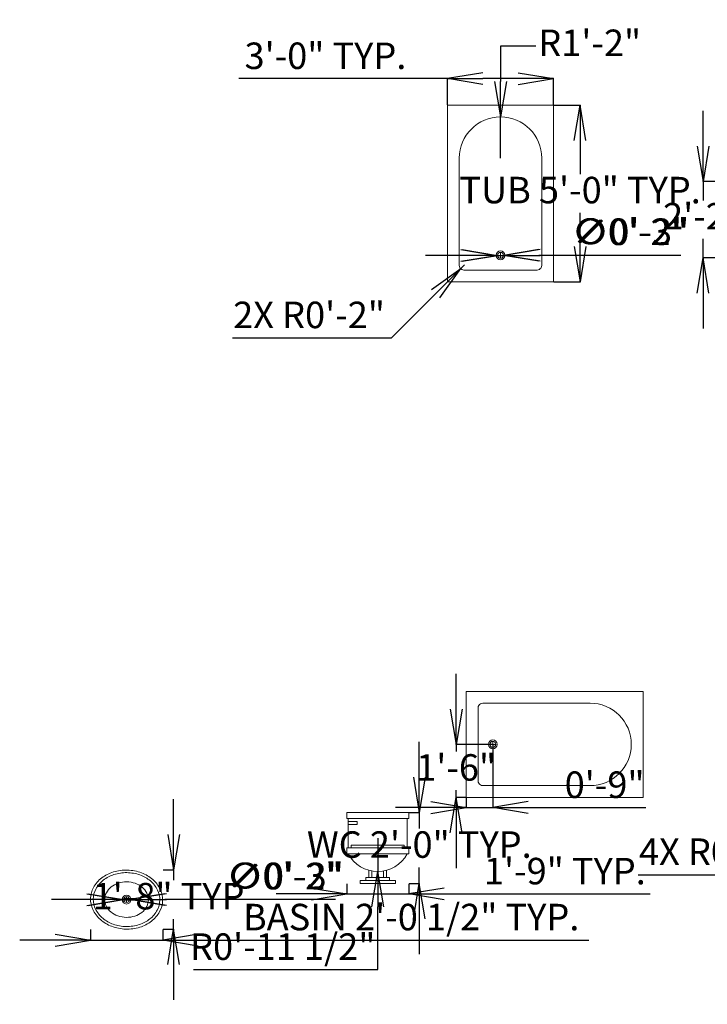
# Model space of a CAD drawing. Units: inches. Extents: x 1856 to 3350, y 1624 to 2224.
# Tile 4 of 7: x 2521 to 2754, y 1634 to 1968. Entities that reach past the tile are written whole.
import ezdxf

# ---------------------------------------------------------------- set-up
doc = ezdxf.new("R2010")
doc.units = ezdxf.units.IN
doc.layers.add('A-ANNO-DIMS', color=2, linetype='Continuous', lineweight=18)
doc.layers.add('A-FLOR-FIXT', color=3, linetype='Continuous', lineweight=18)
doc.styles.get("Standard").update_dxf_attribs({"font": 'arial.ttf'})
doc.dimstyles.new('ISO-25', dxfattribs={"dimtxt": 9, "dimasz": 12, "dimexe": 0.125, "dimexo": 0.125, "dimgap": 2, "dimtad": 1, "dimtih": 1, "dimtoh": 1, "dimdec": 1, "dimzin": 11, "dimlunit": 4, "dimtxsty": 'Standard', "dimblk": 'OPEN', "dimcen": -0.125, "dimadec": 0, "dimazin": 0, "dimtfac": 1, "dimtdec": 1, "dimtmove": 0, "dimatfit": 3, "dimfxl": 1, "dimarcsym": 0})

# ---------------------------------------------------------------- blocks, each defined once
blk = doc.blocks.new('Toilet - front')
for p, q in [((-10, 22), (-10, 12)), ((-10, 21), (-7, 21)), ((-7, 21), (-7, 20)), ((10, 12), (10, 22)), ((-7, 20), (-10, 20)), ((10.5, 12), (-10.5, 12)), ((-10.5, 10), (-10.5, 12)), ((9, 13), (-9, 13)), ((-9, 13), (-9, 12)), ((9, 12), (9, 13)), ((10.5, 12), (10.5, 10)), ((10.5, 10), (-10.5, 10)), ((-3, 4.4065), (-3, 2)), ((-2, 2), (-2, 4.1658)), ((2, 4.1658), (2, 2)), ((3, 2), (3, 4.4065)), ((4, 2), (-4, 2)), ((-4, 2), (-4, 1)), ((4, 1), (4, 2))]:
    blk.add_line(p, q)
for points in [[(10.5, 22), (10.5, 24), (-10.5, 24), (-10.5, 22)], [(6, 0), (6, 1), (-6, 1), (-6, 0)]]:
    blk.add_lwpolyline(points, close=True)
blk.add_arc((0, 15.3333), 11.3333, 208.0725, 331.9275)
blk = doc.blocks.new('Sink - Oval top')
for p, q in [((-1, 0), (1, 0)), ((0, 1), (0, -1))]:
    blk.add_line(p, q)
for points in [[(-12.23, 0.39, 0.117634), (-11.46, -3.36, 0.104469), (-8.88, -6.8, 0.090016), (-5.08, -9.07, 0.08192), (-0.32, -10.02, 0.08192), (4.49, -9.38, 0.090016), (8.42, -7.36, 0.104469), (11.22, -4.09, 0.117634), (12.23, -0.39, 0.117634), (11.46, 3.36, 0.104469), (8.88, 6.8, 0.090016), (5.08, 9.07, 0.08192), (0.32, 10.02, 0.08192), (-4.49, 9.38, 0.090016), (-8.42, 7.36, 0.104469), (-11.22, 4.09, 0.117634)], [(-11.29, 0.16, 0.118622), (-10.52, -3.25, 0.104678), (-8.07, -6.36, 0.089562), (-4.54, -8.37, 0.081185), (-0.13, -9.15, 0.081185), (4.3, -8.49, 0.089562), (7.89, -6.58, 0.104678), (10.42, -3.55, 0.118622), (11.29, -0.16, 0.118622), (10.52, 3.25, 0.104678), (8.07, 6.36, 0.089562), (4.54, 8.37, 0.081185), (0.13, 9.15, 0.081185), (-4.3, 8.49, 0.089562), (-7.89, 6.58, 0.104678), (-10.42, 3.55, 0.118622)], [(-7.42, 0.08, 0.118283), (-6.91, -2.17, 0.104607), (-5.29, -4.21, 0.089718), (-2.97, -5.53, 0.081436), (-0.07, -6.04, 0.081436), (2.84, -5.59, 0.089718), (5.2, -4.33, 0.104607), (6.86, -2.32, 0.118283), (7.42, -0.08, 0.118283), (6.91, 2.17, 0.104607), (5.29, 4.21, 0.089718), (2.97, 5.53, 0.081436), (0.07, 6.04, 0.081436), (-2.84, 5.59, 0.089718), (-5.2, 4.33, 0.104607), (-6.86, 2.32, 0.118283)]]:
    blk.add_lwpolyline(points, format="xyb", close=True)
for radius in [1.5, 1]:
    blk.add_circle((0, 0), radius)
blk = doc.blocks.new('Bath Tub - 26 x 60 in.')
for p, q in [((8, -18), (10, -18)), ((9, -17), (9, -19))]:
    blk.add_line(p, q)
blk.add_lwpolyline([(0, -36), (0, 0), (60, 0), (60, -36)], close=True)
for points in [[(4, -30), (4, -6)], [(6, -4), (42, -4)], [(42, -32), (6, -32)]]:
    blk.add_lwpolyline(points)
for radius in [1.5, 1]:
    blk.add_circle((9, -18), radius)
for centre, radius, start, end in [((5.75, -5.75), 1.77, 81.8699, 188.1301), ((42, -18), 14, 270, 90), ((5.75, -30.25), 1.77, 171.8699, 278.1301)]:
    blk.add_arc(centre, radius, start, end)
blk = doc.blocks.new('_Open')
at = {"color": 0, "linetype": 'ByBlock', "lineweight": -2}
for p, q in [((-1, 0.167), (0, 0)), ((-1, -0.167), (0, 0)), ((0, 0), (-1, 0))]:
    blk.add_line(p, q, dxfattribs=at)
blk = doc.blocks.new('*D50')
at = {"layer": 'A-ANNO-DIMS', "color": 0, "lineweight": -2, "transparency": 16777216}
for p, q in [((2545.08, 1659.26), (2545.08, 1655.58)), ((2569.63, 1659.26), (2569.63, 1655.58)), ((2533.08, 1655.7), (2521.08, 1655.7)), ((2545.08, 1655.7), (2569.63, 1655.7)), ((2581.63, 1655.7), (2714.29, 1655.7))]:
    blk.add_line(p, q, dxfattribs=at)
at = {"layer": 'Defpoints', "color": 0, "transparency": 16777216}
for p in [(2545.08, 1659.39), (2569.63, 1659.39), (2569.63, 1655.7)]:
    blk.add_point(p, dxfattribs=at)
at = {"layer": 'A-ANNO-DIMS', "color": 0, "lineweight": -2, "transparency": 16777216, "xscale": 12, "yscale": 12, "zscale": 12}
blk.add_blockref('_Open', (2545.08, 1655.7), dxfattribs=at)
at = {"layer": 'A-ANNO-DIMS', "color": 0, "lineweight": -2, "transparency": 16777216, "xscale": 12, "yscale": 12, "zscale": 12, "rotation": 180}
blk.add_blockref('_Open', (2569.63, 1655.7), dxfattribs=at)
at = {"layer": 'A-ANNO-DIMS', "color": 0, "transparency": 16777216, "insert": (2653.96, 1662.36), "char_height": 9, "attachment_point": 5}
blk.add_mtext('BASIN 2\'-0 1/2" TYP.', dxfattribs=at)
blk = doc.blocks.new('*D51')
at = {"layer": 'A-ANNO-DIMS', "color": 0, "lineweight": -2, "transparency": 16777216}
for p, q in [((2573.32, 1691.52), (2573.32, 1703.52)), ((2569.76, 1679.52), (2573.44, 1679.52)), ((2573.32, 1679.52), (2573.32, 1676.05)), ((2573.32, 1659.39), (2573.32, 1662.86)), ((2569.76, 1659.39), (2573.44, 1659.39)), ((2573.32, 1647.39), (2573.32, 1635.39))]:
    blk.add_line(p, q, dxfattribs=at)
at = {"layer": 'Defpoints', "color": 0, "transparency": 16777216}
for p in [(2569.63, 1679.52), (2573.32, 1679.52), (2569.63, 1659.39)]:
    blk.add_point(p, dxfattribs=at)
at = {"layer": 'A-ANNO-DIMS', "color": 0, "lineweight": -2, "transparency": 16777216, "xscale": 12, "yscale": 12, "zscale": 12}
for p, rotation in [((2573.32, 1679.52), 270), ((2573.32, 1659.39), 90)]:
    blk.add_blockref('_Open', p, dxfattribs=dict(at, rotation=rotation))
at = {"layer": 'A-ANNO-DIMS', "color": 0, "transparency": 16777216, "insert": (2573.32, 1669.46), "char_height": 9, "attachment_point": 5}
blk.add_mtext('1\'-8" TYP.', dxfattribs=at)
blk = doc.blocks.new('*D52')
at = {"layer": 'A-ANNO-DIMS', "color": 0, "lineweight": -2, "transparency": 16777216}
for p, q in [((2656.73, 1710.98), (2656.73, 1722.98)), ((2653.25, 1698.98), (2656.85, 1698.98)), ((2656.73, 1698.98), (2656.73, 1693.63)), ((2656.73, 1674.98), (2656.73, 1680.32)), ((2653.25, 1674.98), (2656.85, 1674.98)), ((2656.73, 1662.98), (2656.73, 1650.98))]:
    blk.add_line(p, q, dxfattribs=at)
at = {"layer": 'Defpoints', "color": 0, "transparency": 16777216}
for p in [(2653.13, 1698.98), (2656.73, 1698.98), (2653.13, 1674.98)]:
    blk.add_point(p, dxfattribs=at)
at = {"layer": 'A-ANNO-DIMS', "color": 0, "lineweight": -2, "transparency": 16777216, "xscale": 12, "yscale": 12, "zscale": 12}
for p, rotation in [((2656.73, 1698.98), 270), ((2656.73, 1674.98), 90)]:
    blk.add_blockref('_Open', p, dxfattribs=dict(at, rotation=rotation))
at = {"layer": 'A-ANNO-DIMS', "color": 0, "transparency": 16777216, "insert": (2656.73, 1686.98), "char_height": 9, "attachment_point": 5}
blk.add_mtext('WC 2\'-0" TYP.', dxfattribs=at)
blk = doc.blocks.new('*D53')
at = {"layer": 'A-ANNO-DIMS', "color": 0, "lineweight": -2, "transparency": 16777216}
for p, q in [((2632.13, 1674.85), (2632.13, 1671.25)), ((2653.13, 1674.85), (2653.13, 1671.25)), ((2620.13, 1671.38), (2608.13, 1671.38)), ((2632.13, 1671.38), (2653.13, 1671.38)), ((2665.13, 1671.38), (2735.14, 1671.38))]:
    blk.add_line(p, q, dxfattribs=at)
at = {"layer": 'Defpoints', "color": 0, "transparency": 16777216}
for p in [(2632.13, 1674.98), (2653.13, 1674.98), (2653.13, 1671.38)]:
    blk.add_point(p, dxfattribs=at)
at = {"layer": 'A-ANNO-DIMS', "color": 0, "lineweight": -2, "transparency": 16777216, "xscale": 12, "yscale": 12, "zscale": 12}
blk.add_blockref('_Open', (2632.13, 1671.38), dxfattribs=at)
at = {"layer": 'A-ANNO-DIMS', "color": 0, "lineweight": -2, "transparency": 16777216, "xscale": 12, "yscale": 12, "zscale": 12, "rotation": 180}
blk.add_blockref('_Open', (2653.13, 1671.38), dxfattribs=at)
at = {"layer": 'A-ANNO-DIMS', "color": 0, "transparency": 16777216, "insert": (2706.14, 1677.97), "char_height": 9, "attachment_point": 5}
blk.add_mtext('1\'-9" TYP.', dxfattribs=at)
blk = doc.blocks.new('*D54')
at = {"layer": 'A-ANNO-DIMS', "color": 0, "lineweight": -2, "transparency": 16777216}
for p, q in [((2702.42, 1939.19), (2711.42, 1939.19)), ((2711.3, 1927.19), (2711.3, 1915.79)), ((2711.3, 1891.19), (2711.3, 1902.59)), ((2702.42, 1879.19), (2711.42, 1879.19))]:
    blk.add_line(p, q, dxfattribs=at)
at = {"layer": 'Defpoints', "color": 0, "transparency": 16777216}
for p in [(2702.3, 1939.19), (2711.3, 1939.19), (2702.3, 1879.19)]:
    blk.add_point(p, dxfattribs=at)
at = {"layer": 'A-ANNO-DIMS', "color": 0, "lineweight": -2, "transparency": 16777216, "xscale": 12, "yscale": 12, "zscale": 12}
for p, rotation in [((2711.3, 1939.19), 90), ((2711.3, 1879.19), 270)]:
    blk.add_blockref('_Open', p, dxfattribs=dict(at, rotation=rotation))
at = {"layer": 'A-ANNO-DIMS', "color": 0, "transparency": 16777216, "insert": (2711.3, 1909.19), "char_height": 9, "attachment_point": 5}
blk.add_mtext('TUB 5\'-0" TYP.', dxfattribs=at)
blk = doc.blocks.new('*D55')
at = {"layer": 'A-ANNO-DIMS', "color": 0, "lineweight": -2, "transparency": 16777216}
for p, q in [((2666.3, 1948.19), (2595.44, 1948.19)), ((2666.3, 1939.31), (2666.3, 1948.31)), ((2690.3, 1948.19), (2678.3, 1948.19)), ((2702.3, 1939.31), (2702.3, 1948.31))]:
    blk.add_line(p, q, dxfattribs=at)
at = {"layer": 'Defpoints', "color": 0, "transparency": 16777216}
for p in [(2666.3, 1948.19), (2666.3, 1939.19), (2702.3, 1939.19)]:
    blk.add_point(p, dxfattribs=at)
at = {"layer": 'A-ANNO-DIMS', "color": 0, "lineweight": -2, "transparency": 16777216, "xscale": 12, "yscale": 12, "zscale": 12, "rotation": 180}
blk.add_blockref('_Open', (2666.3, 1948.19), dxfattribs=at)
at = {"layer": 'A-ANNO-DIMS', "color": 0, "lineweight": -2, "transparency": 16777216, "xscale": 12, "yscale": 12, "zscale": 12}
blk.add_blockref('_Open', (2702.3, 1948.19), dxfattribs=at)
at = {"layer": 'A-ANNO-DIMS', "color": 0, "transparency": 16777216, "insert": (2624.87, 1954.79), "char_height": 9, "attachment_point": 5}
blk.add_mtext('3\'-0" TYP.', dxfattribs=at)
blk = doc.blocks.new('*D76')
at = {"layer": 'A-ANNO-DIMS', "color": 0, "lineweight": -2, "transparency": 16777216}
for p, q in [((2753.05, 1925.32), (2753.05, 1937.32)), ((2757.48, 1913.32), (2752.93, 1913.32)), ((2753.05, 1913.32), (2753.05, 1906.83)), ((2753.05, 1887.32), (2753.05, 1893.8)), ((2757.48, 1887.32), (2752.93, 1887.32)), ((2753.05, 1875.32), (2753.05, 1863.32))]:
    blk.add_line(p, q, dxfattribs=at)
at = {"layer": 'Defpoints', "color": 0, "transparency": 16777216}
for p in [(2757.6, 1913.32), (2753.05, 1887.32), (2757.6, 1887.32)]:
    blk.add_point(p, dxfattribs=at)
at = {"layer": 'A-ANNO-DIMS', "color": 0, "lineweight": -2, "transparency": 16777216, "xscale": 12, "yscale": 12, "zscale": 12}
for p, rotation in [((2753.05, 1913.32), 270), ((2753.05, 1887.32), 90)]:
    blk.add_blockref('_Open', p, dxfattribs=dict(at, rotation=rotation))
at = {"layer": 'A-ANNO-DIMS', "color": 0, "transparency": 16777216, "insert": (2753.05, 1900.32), "char_height": 9, "attachment_point": 5}
blk.add_mtext('2\'-2"', dxfattribs=at)
blk = doc.blocks.new('*D87')
at = {"layer": 'A-ANNO-DIMS', "color": 0, "lineweight": -2, "transparency": 16777216}
for p, q in [((2681.68, 1722.03), (2681.68, 1700.58)), ((2672.68, 1704.03), (2672.68, 1700.58)), ((2660.68, 1700.71), (2648.68, 1700.71)), ((2672.68, 1700.71), (2681.68, 1700.71)), ((2693.68, 1700.71), (2733.6, 1700.71))]:
    blk.add_line(p, q, dxfattribs=at)
at = {"layer": 'Defpoints', "color": 0, "transparency": 16777216}
for p in [(2681.68, 1722.16), (2672.68, 1704.16), (2681.68, 1700.71)]:
    blk.add_point(p, dxfattribs=at)
at = {"layer": 'A-ANNO-DIMS', "color": 0, "lineweight": -2, "transparency": 16777216, "xscale": 12, "yscale": 12, "zscale": 12}
blk.add_blockref('_Open', (2672.68, 1700.71), dxfattribs=at)
at = {"layer": 'A-ANNO-DIMS', "color": 0, "lineweight": -2, "transparency": 16777216, "xscale": 12, "yscale": 12, "zscale": 12, "rotation": 180}
blk.add_blockref('_Open', (2681.68, 1700.71), dxfattribs=at)
at = {"layer": 'A-ANNO-DIMS', "color": 0, "transparency": 16777216, "insert": (2719.64, 1707.3), "char_height": 9, "attachment_point": 5}
blk.add_mtext('0\'-9"', dxfattribs=at)
blk = doc.blocks.new('*D88')
at = {"layer": 'A-ANNO-DIMS', "color": 0, "lineweight": -2, "transparency": 16777216}
for p, q in [((2669.23, 1734.16), (2669.23, 1746.16)), ((2681.55, 1722.16), (2669.1, 1722.16)), ((2669.23, 1722.16), (2669.23, 1719.75)), ((2669.23, 1704.16), (2669.23, 1706.56)), ((2672.55, 1704.16), (2669.1, 1704.16)), ((2669.23, 1692.16), (2669.23, 1680.16))]:
    blk.add_line(p, q, dxfattribs=at)
at = {"layer": 'Defpoints', "color": 0, "transparency": 16777216}
for p in [(2669.23, 1722.16), (2681.68, 1722.16), (2672.68, 1704.16)]:
    blk.add_point(p, dxfattribs=at)
at = {"layer": 'A-ANNO-DIMS', "color": 0, "lineweight": -2, "transparency": 16777216, "xscale": 12, "yscale": 12, "zscale": 12}
for p, rotation in [((2669.23, 1722.16), 270), ((2669.23, 1704.16), 90)]:
    blk.add_blockref('_Open', p, dxfattribs=dict(at, rotation=rotation))
at = {"layer": 'A-ANNO-DIMS', "color": 0, "transparency": 16777216, "insert": (2669.23, 1713.16), "char_height": 9, "attachment_point": 5}
blk.add_mtext('1\'-6"', dxfattribs=at)
blk = doc.blocks.new('*D101')
at = {"layer": 'A-ANNO-DIMS', "color": 0, "lineweight": -2, "transparency": 16777216}
for p, q in [((2830.88, 1702.51), (2829.82, 1701.45)), ((2806.26, 1677.9), (2821.33, 1692.97)), ((2731.06, 1677.9), (2806.26, 1677.9))]:
    blk.add_line(p, q, dxfattribs=at)
at = {"layer": 'Defpoints', "color": 0, "transparency": 16777216}
for p in [(2830.88, 1702.51), (2829.82, 1701.45)]:
    blk.add_point(p, dxfattribs=at)
at = {"layer": 'A-ANNO-DIMS', "color": 0, "lineweight": -2, "transparency": 16777216, "xscale": 12, "yscale": 12, "zscale": 12, "rotation": 44.99157303797349}
blk.add_blockref('_Open', (2829.82, 1701.45), dxfattribs=at)
at = {"layer": 'A-ANNO-DIMS', "color": 0, "transparency": 16777216, "insert": (2767.66, 1684.56), "char_height": 9, "attachment_point": 5}
blk.add_mtext('4X R0\'-1 1/2"', dxfattribs=at)
blk = doc.blocks.new('*D102')
at = {"layer": 'A-ANNO-DIMS', "color": 0, "lineweight": -2, "transparency": 16777216}
for p, q in [((2696.3, 1959.19), (2684.3, 1959.19)), ((2684.3, 1959.19), (2684.3, 1947.19)), ((2684.3, 1921.19), (2684.3, 1935.19))]:
    blk.add_line(p, q, dxfattribs=at)
at = {"layer": 'Defpoints', "color": 0, "transparency": 16777216}
for p in [(2684.3, 1935.19), (2684.3, 1921.19)]:
    blk.add_point(p, dxfattribs=at)
at = {"layer": 'A-ANNO-DIMS', "color": 0, "lineweight": -2, "transparency": 16777216, "xscale": 12, "yscale": 12, "zscale": 12, "rotation": 269.9990218791928}
blk.add_blockref('_Open', (2684.3, 1935.19), dxfattribs=at)
at = {"layer": 'A-ANNO-DIMS', "color": 0, "transparency": 16777216, "insert": (2714.57, 1959.19), "char_height": 9, "attachment_point": 5}
blk.add_mtext('R1\'-2"', dxfattribs=at)
blk = doc.blocks.new('*D103')
at = {"layer": 'A-ANNO-DIMS', "color": 0, "lineweight": -2, "transparency": 16777216}
for p, q in [((2672.05, 1884.94), (2670.8, 1883.69)), ((2647.33, 1860.22), (2662.31, 1875.2)), ((2593.3, 1860.22), (2647.33, 1860.22))]:
    blk.add_line(p, q, dxfattribs=at)
at = {"layer": 'Defpoints', "color": 0, "transparency": 16777216}
for p in [(2670.8, 1883.69), (2672.05, 1884.94)]:
    blk.add_point(p, dxfattribs=at)
at = {"layer": 'A-ANNO-DIMS', "color": 0, "lineweight": -2, "transparency": 16777216, "xscale": 12, "yscale": 12, "zscale": 12, "rotation": 45.00288770727251}
blk.add_blockref('_Open', (2670.8, 1883.69), dxfattribs=at)
at = {"layer": 'A-ANNO-DIMS', "color": 0, "transparency": 16777216, "insert": (2619.31, 1866.81), "char_height": 9, "attachment_point": 5}
blk.add_mtext('2X R0\'-2"', dxfattribs=at)
blk = doc.blocks.new('*D104')
at = {"layer": 'A-ANNO-DIMS', "color": 0, "lineweight": -2, "transparency": 16777216}
for p, q in [((2670.8, 1888.19), (2658.8, 1888.19)), ((2682.8, 1888.19), (2685.8, 1888.19)), ((2709.8, 1888.19), (2697.8, 1888.19)), ((2745.51, 1888.19), (2709.8, 1888.19))]:
    blk.add_line(p, q, dxfattribs=at)
at = {"layer": 'Defpoints', "color": 0, "transparency": 16777216}
for p in [(2682.8, 1888.19), (2685.8, 1888.19)]:
    blk.add_point(p, dxfattribs=at)
at = {"layer": 'A-ANNO-DIMS', "color": 0, "lineweight": -2, "transparency": 16777216, "xscale": 12, "yscale": 12, "zscale": 12}
for p, rotation in [((2682.8, 1888.19), 0.0043162820506559), ((2685.8, 1888.19), 180.0043162820506)]:
    blk.add_blockref('_Open', p, dxfattribs=dict(at, rotation=rotation))
at = {"layer": 'A-ANNO-DIMS', "color": 0, "transparency": 16777216, "insert": (2728.65, 1895.04), "char_height": 9, "attachment_point": 5}
blk.add_mtext('∅0\'-3"', dxfattribs=at)
blk = doc.blocks.new('*D105')
at = {"layer": 'A-ANNO-DIMS', "color": 0, "lineweight": -2, "transparency": 16777216}
for p, q in [((2671.3, 1888.19), (2659.3, 1888.19)), ((2683.3, 1888.19), (2685.3, 1888.19)), ((2709.3, 1888.19), (2697.3, 1888.19)), ((2745.01, 1888.19), (2709.3, 1888.19))]:
    blk.add_line(p, q, dxfattribs=at)
at = {"layer": 'Defpoints', "color": 0, "transparency": 16777216}
for p in [(2683.3, 1888.19), (2685.3, 1888.19)]:
    blk.add_point(p, dxfattribs=at)
at = {"layer": 'A-ANNO-DIMS', "color": 0, "lineweight": -2, "transparency": 16777216, "xscale": 12, "yscale": 12, "zscale": 12}
for p, rotation in [((2683.3, 1888.19), 0.0064744230541614), ((2685.3, 1888.19), 180.0064744230541)]:
    blk.add_blockref('_Open', p, dxfattribs=dict(at, rotation=rotation))
at = {"layer": 'A-ANNO-DIMS', "color": 0, "transparency": 16777216, "insert": (2728.15, 1895.04), "char_height": 9, "attachment_point": 5}
blk.add_mtext('∅0\'-2"', dxfattribs=at)
blk = doc.blocks.new('*D106')
at = {"layer": 'A-ANNO-DIMS', "color": 0, "lineweight": -2, "transparency": 16777216}
for p, q in [((2642.63, 1690.31), (2642.63, 1678.98)), ((2642.63, 1645.67), (2642.63, 1666.98)), ((2580.13, 1645.67), (2642.63, 1645.67))]:
    blk.add_line(p, q, dxfattribs=at)
at = {"layer": 'Defpoints', "color": 0, "transparency": 16777216}
for p in [(2642.63, 1690.31), (2642.63, 1678.98)]:
    blk.add_point(p, dxfattribs=at)
at = {"layer": 'A-ANNO-DIMS', "color": 0, "lineweight": -2, "transparency": 16777216, "xscale": 12, "yscale": 12, "zscale": 12, "rotation": 89.99933267248882}
blk.add_blockref('_Open', (2642.63, 1678.98), dxfattribs=at)
at = {"layer": 'A-ANNO-DIMS', "color": 0, "transparency": 16777216, "insert": (2610.38, 1652.32), "char_height": 9, "attachment_point": 5}
blk.add_mtext('R0\'-11 1/2"', dxfattribs=at)
blk = doc.blocks.new('*D107')
at = {"layer": 'A-ANNO-DIMS', "color": 0, "lineweight": -2, "transparency": 16777216}
for p, q in [((2543.86, 1669.46), (2531.86, 1669.46)), ((2555.86, 1669.46), (2558.86, 1669.45)), ((2592.55, 1669.45), (2570.86, 1669.45)), ((2628.27, 1669.45), (2592.55, 1669.45))]:
    blk.add_line(p, q, dxfattribs=at)
at = {"layer": 'Defpoints', "color": 0, "transparency": 16777216}
for p in [(2555.86, 1669.46), (2558.86, 1669.45)]:
    blk.add_point(p, dxfattribs=at)
at = {"layer": 'A-ANNO-DIMS', "color": 0, "lineweight": -2, "transparency": 16777216, "xscale": 12, "yscale": 12, "zscale": 12}
for p, rotation in [((2555.86, 1669.46), 359.985752449785), ((2558.86, 1669.45), 179.9857524497849)]:
    blk.add_blockref('_Open', p, dxfattribs=dict(at, rotation=rotation))
at = {"layer": 'A-ANNO-DIMS', "color": 0, "transparency": 16777216, "insert": (2611.41, 1676.29), "char_height": 9, "attachment_point": 5}
blk.add_mtext('∅0\'-3"', dxfattribs=at)
blk = doc.blocks.new('*D108')
at = {"layer": 'A-ANNO-DIMS', "color": 0, "lineweight": -2, "transparency": 16777216}
for p, q in [((2544.36, 1669.46), (2532.36, 1669.46)), ((2556.36, 1669.46), (2558.36, 1669.45)), ((2592.05, 1669.44), (2570.36, 1669.45)), ((2627.77, 1669.44), (2592.05, 1669.44))]:
    blk.add_line(p, q, dxfattribs=at)
at = {"layer": 'Defpoints', "color": 0, "transparency": 16777216}
for p in [(2556.36, 1669.46), (2558.36, 1669.45)]:
    blk.add_point(p, dxfattribs=at)
at = {"layer": 'A-ANNO-DIMS', "color": 0, "lineweight": -2, "transparency": 16777216, "xscale": 12, "yscale": 12, "zscale": 12}
for p, rotation in [((2556.36, 1669.46), 359.9786286752216), ((2558.36, 1669.45), 179.9786286752215)]:
    blk.add_blockref('_Open', p, dxfattribs=dict(at, rotation=rotation))
at = {"layer": 'A-ANNO-DIMS', "color": 0, "transparency": 16777216, "insert": (2610.91, 1676.29), "char_height": 9, "attachment_point": 5}
blk.add_mtext('∅0\'-2"', dxfattribs=at)

msp = doc.modelspace()

# ---------------------------------------------------------------- block references
at = {"layer": 'A-FLOR-FIXT', "rotation": 90}
msp.add_blockref('Bath Tub - 26 x 60 in.', (2666.3, 1879.19), dxfattribs=at)
at = {"layer": 'A-FLOR-FIXT'}
for name, p in [('Bath Tub - 26 x 60 in.', (2672.68, 1740.16)), ('Toilet - front', (2642.63, 1674.98)), ('Sink - Oval top', (2557.36, 1669.46))]:
    msp.add_blockref(name, p, dxfattribs=at)

# ---------------------------------------------------------------- dimensions: what is measured, and where the dimension line sits
at = {"layer": 'A-ANNO-DIMS'}
for base, p1, p2, angle, text, picture, middle in [((2666.3, 1948.19), (2702.3, 1939.19), (2666.3, 1939.19), 180, '<> TYP.', '*D55', (2624.87, 1954.79)), ((2711.3, 1939.19), (2702.3, 1879.19), (2702.3, 1939.19), 90, 'TUB <> TYP.', '*D54', (2711.3, 1909.19)), ((2656.73, 1698.98), (2653.13, 1674.98), (2653.13, 1698.98), 90, 'WC <> TYP.', '*D52', (2656.73, 1686.98)), ((2573.32, 1679.52), (2569.63, 1659.39), (2569.63, 1679.52), 90, '<> TYP.', '*D51', (2573.32, 1669.46))]:
    dim = msp.add_linear_dim(base=base, p1=p1, p2=p2, angle=angle, text=text, dimstyle='ISO-25', override={"dimdec": 1, "dimlfac": 1, "dimrnd": 0, "dimzin": 1, "dimdsep": 46, "dimlunit": 4, "dimfrac": 2}, dxfattribs=at)
    dim.commit()
    dim.dimension.update_dxf_attribs({"geometry": picture, "text_midpoint": middle})
for center, mpoint, picture, middle in [((2684.3, 1921.19), (2684.3, 1935.19), '*D102', (2714.57, 1959.19)), ((2642.63, 1690.31), (2642.63, 1678.98), '*D106', (2610.38, 1652.32))]:
    dim = msp.add_radius_dim(center=center, mpoint=mpoint, dimstyle='ISO-25', override={"dimdec": 1, "dimlfac": 1, "dimrnd": 0, "dimzin": 1, "dimdsep": 46, "dimlunit": 4, "dimfrac": 2}, dxfattribs=at)
    dim.commit()
    dim.dimension.update_dxf_attribs({"geometry": picture, "text_midpoint": middle})
for base, p1, p2, picture, middle in [((2753.05, 1887.32), (2757.6, 1913.32), (2757.6, 1887.32), '*D76', (2753.05, 1900.32)), ((2669.23, 1722.16), (2672.68, 1704.16), (2681.68, 1722.16), '*D88', (2669.23, 1713.16))]:
    dim = msp.add_linear_dim(base=base, p1=p1, p2=p2, angle=90, dimstyle='ISO-25', override={"dimdec": 1, "dimlfac": 1, "dimrnd": 0, "dimzin": 1, "dimdsep": 46, "dimlunit": 4, "dimfrac": 2}, dxfattribs=at)
    dim.commit()
    dim.dimension.update_dxf_attribs({"geometry": picture, "text_midpoint": middle})
dim = msp.add_diameter_dim_2p(p1=(2682.8, 1888.19), p2=(2685.8, 1888.19), dimstyle='ISO-25', override={"dimdec": 1, "dimlfac": 1, "dimrnd": 0, "dimzin": 1, "dimdsep": 46, "dimlunit": 4, "dimfrac": 2}, dxfattribs=at)
dim.commit()
dim.dimension.update_dxf_attribs({"geometry": '*D104', "text_midpoint": (2709.8, 1888.19), "dimtype": 163})
for p1, p2, picture, middle in [((2683.3, 1888.19), (2685.3, 1888.19), '*D105', (2709.3, 1888.19)), ((2555.86, 1669.46), (2558.86, 1669.45), '*D107', (2592.55, 1669.45)), ((2556.36, 1669.46), (2558.36, 1669.45), '*D108', (2592.05, 1669.44))]:
    dim = msp.add_diameter_dim_2p(p1=p1, p2=p2, dimstyle='ISO-25', override={"dimdec": 1, "dimlfac": 1, "dimrnd": 0, "dimzin": 1, "dimdsep": 46, "dimlunit": 4, "dimfrac": 2}, dxfattribs=at)
    dim.commit()
    dim.dimension.update_dxf_attribs({"geometry": picture, "text_midpoint": middle})
for center, mpoint, text, picture, middle in [((2672.05, 1884.94), (2670.8, 1883.69), '2X <>', '*D103', (2619.31, 1866.81)), ((2830.88, 1702.51), (2829.82, 1701.45), '4X <>', '*D101', (2767.66, 1684.56))]:
    dim = msp.add_radius_dim(center=center, mpoint=mpoint, text=text, dimstyle='ISO-25', override={"dimdec": 1, "dimlfac": 1, "dimrnd": 0, "dimzin": 1, "dimdsep": 46, "dimlunit": 4, "dimfrac": 2}, dxfattribs=at)
    dim.commit()
    dim.dimension.update_dxf_attribs({"geometry": picture, "text_midpoint": middle})
dim = msp.add_linear_dim(base=(2681.68, 1700.71), p1=(2672.68, 1704.16), p2=(2681.68, 1722.16), dimstyle='ISO-25', override={"dimdec": 1, "dimlfac": 1, "dimrnd": 0, "dimzin": 1, "dimdsep": 46, "dimlunit": 4, "dimfrac": 2}, dxfattribs=at)
dim.commit()
dim.dimension.update_dxf_attribs({"geometry": '*D87', "text_midpoint": (2719.64, 1707.3)})
for base, p1, p2, text, picture, middle in [((2569.6334, 1655.7044), (2545.0825, 1659.3871), (2569.6334, 1659.3871), 'BASIN <> TYP.', '*D50', (2653.9615, 1662.3579)), ((2653.13, 1671.38), (2632.13, 1674.98), (2653.13, 1674.98), '<> TYP.', '*D53', (2706.14, 1677.97))]:
    dim = msp.add_linear_dim(base=base, p1=p1, p2=p2, text=text, dimstyle='ISO-25', override={"dimdec": 1, "dimlfac": 1, "dimrnd": 0, "dimzin": 1, "dimdsep": 46, "dimlunit": 4, "dimfrac": 2}, dxfattribs=at)
    dim.commit()
    dim.dimension.update_dxf_attribs({"geometry": picture, "text_midpoint": middle})

doc.saveas('drawing.dxf')
